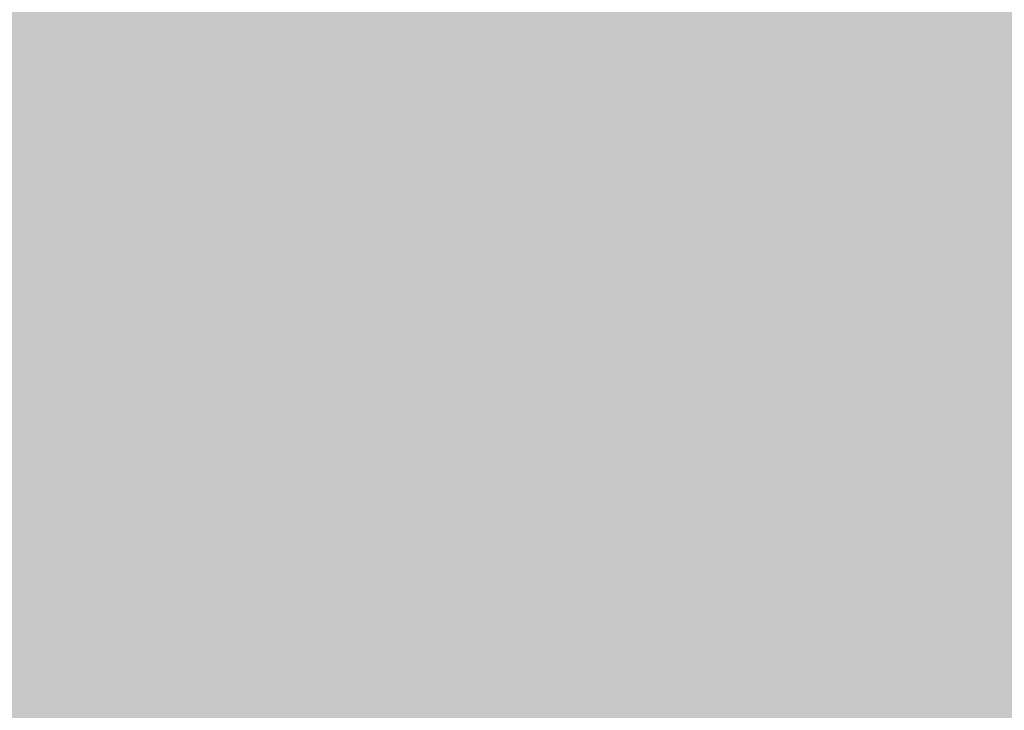
# Model space of a CAD drawing. Units: inches. Extents: x 2091 to 2899, y 967 to 2217.
# Tile 171 of 256: x 2203.14684 to 2203.151632, y 1152.250422 to 1152.253784. Entities that reach past the tile are written whole.
import ezdxf

# ---------------------------------------------------------------- set-up
doc = ezdxf.new("R2010")
doc.units = ezdxf.units.IN
doc.layers.add('A-WALL-PATT', color=141, linetype='Continuous', lineweight=13, true_color=0xadddf7)

msp = doc.modelspace()

# ---------------------------------------------------------------- hatches: boundary and pattern name
at = {"layer": 'A-WALL-PATT'}
h = msp.add_hatch(color=256, dxfattribs=at)
h.dxf.hatch_style = 1
h.paths.add_polyline_path([(2803.1436027, 2050.9190588), (2203.1436027, 2050.9190588), (2203.1436027, 1090.9190588), (2803.1436027, 1090.9190588)])
h.paths.add_polyline_path([(2635.7988501, 1147.5404649), (2674.5240524, 1147.5404649, 0.376086), (2678.5296653, 1152.8802017), (2678.5296653, 1159.5564734, 0.333335), (2674.524319, 1163.561846), (2674.524319, 1163.5618504), (2674.524319, 1192.9343904), (2635.8059707, 1192.9343904), (2597.0876225, 1192.9343904), (2597.0876225, 1163.561846, 0.333335), (2593.0822761, 1159.5564734), (2593.0822761, 1152.8802017, 0.376086), (2597.087889, 1147.5404649)], flags=0)
h.paths.add_polyline_path([(2436.0104329, 1278.2407784, 0.000483), (2435.9526433, 1278.215027, -0.001328), (2435.9356253, 1278.1116934, -0.001711), (2436.1164401, 1278.0407583, 0.002185)], flags=0)
h.paths.add_polyline_path([(2794.1436027, 1143.4190588), (2794.1436027, 1347.4190588), (2543.3701706, 1347.4190588), (2543.3701706, 1351.9190588), (2794.1436027, 1351.9190588), (2794.1436027, 1392.7135549), (2793.9473982, 1392.7135549), (2793.9473982, 1473.5368999), (2794.1436027, 1473.5368999), (2794.1436027, 1531.9190588), (2650.1436027, 1531.9190588), (2650.1436027, 1536.4190588), (2794.1436027, 1536.4190588), (2794.1436027, 1692.4190588), (2609.3756095, 1692.4190588), (2609.3756095, 1644.4190588), (2604.8756095, 1644.4190588), (2604.8756095, 1744.9190588), (2609.3756095, 1744.9190588), (2609.3756095, 1696.9190588), (2794.1436027, 1696.9190588), (2794.1436027, 1780.9190588), (2609.6436027, 1780.9190588), (2493.8756095, 1780.9190588), (2493.8756095, 1785.4190588), (2609.6436027, 1785.4190588), (2794.1436027, 1785.4190588), (2794.1436027, 1847.9388214), (2793.9512217, 1847.9388214), (2793.9512217, 1928.7621663), (2794.1436027, 1928.7621663), (2794.1436027, 1941.4190588), (2614.1436027, 1941.4190588), (2614.1436027, 1821.4190588), (2609.6436027, 1821.4190588), (2609.6436027, 1941.4190588), (2392.1436027, 1941.4190588), (2392.1436027, 1819.9190588), (2387.6436027, 1819.9190588), (2387.6436027, 1941.4190588), (2212.1436027, 1941.4190588), (2212.1436027, 1783.9190588), (2392.1436027, 1783.9190588), (2392.1436027, 1780.9190588), (2212.1436027, 1780.9190588), (2212.1436027, 1629.4190588), (2387.6436027, 1629.4190588), (2387.6436027, 1744.9190588), (2392.1436027, 1744.9190588), (2392.1436027, 1627.9190588), (2317.1436027, 1627.9190588), (2317.1436027, 1551.4190588), (2317.1436027, 1536.4190588), (2459.3835909, 1536.4190588), (2459.3835909, 1602.3964802), (2463.8835909, 1602.3964802), (2463.8835909, 1531.9190588), (2456.6436027, 1531.9190588), (2456.6436027, 1529.9190588), (2452.1436027, 1529.9190588), (2452.1436027, 1531.9190588), (2312.6436027, 1531.9190588), (2312.6436027, 1551.4190588), (2306.1436027, 1551.4190588), (2306.1436027, 1555.9190588), (2308.1436027, 1555.9190588), (2308.1436027, 1551.4190588), (2312.6436027, 1551.4190588), (2312.6436027, 1627.9190588), (2212.1436027, 1627.9190588), (2212.1436027, 1555.9190588), (2270.1436027, 1555.9190588), (2270.1436027, 1551.4190588), (2212.1436027, 1551.4190588), (2212.1436027, 1351.9190588), (2272.1436027, 1351.9190588), (2272.1436027, 1347.4190588), (2212.1436027, 1347.4190588), (2212.1436027, 1275.4190588), (2308.1436027, 1275.4190588), (2308.1436027, 1351.9190588), (2452.1436027, 1351.9190588), (2452.1436027, 1493.9190588), (2456.6436027, 1493.9190588), (2456.6436027, 1347.4190588), (2312.6436027, 1347.4190588), (2312.6436027, 1270.9190588), (2212.1436027, 1270.9190588), (2212.1436027, 1099.9190588), (2281.2375229, 1099.9190588), (2282.8710413, 1110.9138034), (2282.0083413, 1116.9966034), (2278.5577413, 1121.4204034), (2268.2056413, 1128.0562034), (2272.0876413, 1128.0562034), (2273.8129413, 1131.9270034), (2279.4203413, 1134.6919034), (2285.0278413, 1135.2449034), (2287.6158413, 1137.4568034), (2288.0471413, 1138.0098034), (2289.3411413, 1140.7747034), (2291.0665413, 1139.6687034), (2292.3605413, 1135.2449034), (2295.3798413, 1136.9038034), (2296.2425413, 1135.7979034), (2297.1052413, 1133.0330034), (2300.1246413, 1138.0098034), (2303.1439413, 1138.0098034), (2304.4379413, 1135.7979034), (2303.1439413, 1133.5860034), (2306.5946413, 1134.6919034), (2307.8887413, 1133.0330034), (2310.9080413, 1135.2449034), (2313.9274413, 1134.1389034), (2315.6268599, 1132.4271023), (2308.3200413, 1117.5496034), (2290.2038413, 1109.8079034), (2288.9098413, 1103.1721034), (2289.2723086, 1099.9190588), (2434.9182274, 1099.9190588), (2431.5932274, 1124.7880588), (2429.9302274, 1169.5530588), (2430.9271848, 1240.5196942), (2435.6589255, 1238.1861258), (2437.1352274, 1196.5540588), (2438.7982274, 1143.9730588), (2442.6782274, 1111.9980588), (2446.5582274, 1099.9190588), (2794.1436027, 1099.9190588), (2794.1436027, 1138.9190588), (2548.0324471, 1138.9190588), (2548.0324471, 1143.4190588), (2548.0324471, 1148.8190588), (2546.6684571, 1148.0315588), (2528.6856919, 1179.1786218, 0.256256), (2512.0324471, 1148.8190588), (2512.0324471, 1143.4190588), (2512.0324471, 1138.9190588), (2507.5324471, 1138.9190588), (2507.5324471, 1143.4190588), (2507.5324471, 1148.8190588, 0.256256), (2490.8792023, 1179.1786218), (2472.8964371, 1148.0315588), (2471.5324471, 1148.8190588), (2471.5324471, 1143.4190588), (2467.0324471, 1143.4190588), (2467.0324471, 1269.9457858, 0.039061), (2460.9099871, 1273.5800588), (2467.0324471, 1273.5800588), (2467.0324471, 1286.3253638, 0.014511), (2465.2161944, 1286.7619052), (2467.0324471, 1287.0525761), (2467.0324471, 1323.4190588), (2471.5324471, 1323.4190588), (2471.5324471, 1148.8190588), (2489.5324471, 1179.9959734), (2490.8964371, 1179.2084734), (2490.8792023, 1179.1786218, -0.256256), (2507.5324471, 1148.8190588), (2507.5324471, 1143.4190588), (2512.0324471, 1143.4190588), (2512.0324471, 1148.8190588, -0.256256), (2528.6856919, 1179.1786218), (2528.6684571, 1179.2084734), (2530.0324471, 1179.9959734), (2548.0324471, 1148.8190588), (2548.0324471, 1143.4190588)], flags=16)
h.paths.add_polyline_path([(2607.7685461, 1200.9450832), (2607.7685461, 1265.0306251), (2597.0876225, 1281.0520106), (2619.7845852, 1281.0520106), (2627.795278, 1337.1268598), (2635.7988501, 1337.1268598), (2643.8166634, 1337.1268598), (2651.8273562, 1281.0520106), (2674.524319, 1281.0520106), (2663.8433953, 1265.0306251), (2663.8433953, 1200.9450832), (2635.8059707, 1200.9450832)], flags=0)
edge = h.paths.add_edge_path(flags=0)
edge.add_ellipse((13303.8962153, 1272.9987247), major_axis=(-10595.3130399, 0.0000005), ratio=0.842303870086, start_angle=0.62823721906, end_angle=0.64655409989, ccw=False)
edge.add_ellipse((2711.7004495, 1156.8526781), major_axis=(2.2197691, 0), ratio=0.84230387, start_angle=111.5352435, end_angle=180.6282372, ccw=False)
edge.add_ellipse((13303.1562922, 1272.9987246), major_axis=(-10593.0263064, 0), ratio=0.842303869544, start_angle=0.52827147182, end_angle=0.64655409706, ccw=False)
edge.add_line((2710.7645961, 1175.3332951), (2710.1299858, 1175.3332951))
edge.add_ellipse((2710.1299858, 1176.5797752), major_axis=(1.4798461, 0), ratio=0.84230387, start_angle=180, end_angle=270, ccw=False)
edge.add_line((2708.6501397, 1176.5797752), (2708.6501397, 1200.7829144))
edge.add_ellipse((2710.1299858, 1200.7829144), major_axis=(1.4798461, 0), ratio=0.84230387, start_angle=90, end_angle=180, ccw=False)
edge.add_line((2710.1299858, 1202.0293944), (2710.4650752, 1202.0293944))
edge.add_ellipse((13303.1562922, 1272.9987246), major_axis=(-10593.0263064, 0), ratio=0.842303869544, start_angle=-0.09022908859, end_angle=0.38386677879, ccw=False)
edge.add_ellipse((2710.1299858, 1290.9270308), major_axis=(-1.4798461, 0), ratio=0.84230387, start_angle=0, end_angle=90, ccw=False)
edge.add_line((2708.6501397, 1290.9270308), (2708.6501397, 1315.13017))
edge.add_ellipse((2710.1299858, 1315.13017), major_axis=(-1.4798461, 0), ratio=0.84230387, start_angle=-90, end_angle=0, ccw=False)
edge.add_line((2710.1299858, 1316.3766501), (2710.7063141, 1316.3766501))
edge.add_ellipse((3238.4017202, 1296.2895655), major_axis=(528.2339998, 0), ratio=0.84230386954, start_angle=176.349572414, end_angle=177.820049686, ccw=False)
edge.add_ellipse((2775.0630432, 1071.4506962), major_axis=(313.3077613, 0), ratio=0.84230386954, start_angle=102.125965552, end_angle=103.780528989, ccw=False)
edge.add_ellipse((2775.0630432, 1078.3056979), major_axis=(-305.3028915, 0), ratio=0.84230386955, start_angle=-79.790461003, end_angle=-77.555372706, ccw=False)
edge.add_ellipse((2695.1417666, 1541.9753825), major_axis=(-250.9602162, 0), ratio=0.84230386954, start_angle=99.256566007, end_angle=102.554932644)
edge.add_line((2741.4103262, 1334.2142554), (2747.1325454, 1337.3784768))
edge.add_ellipse((2747.5386163, 1336.8574776), major_axis=(-0.739923, 0), ratio=0.84230387, start_angle=270, end_angle=307.9331305, ccw=False)
edge.add_ellipse((2747.5386163, 1336.8574776), major_axis=(-0.739923, 0), ratio=0.84230387, start_angle=232.0668695, end_angle=270, ccw=False)
edge.add_line((2747.9446872, 1337.3784768), (2753.6669064, 1334.2142554))
edge.add_ellipse((2799.935466, 1541.9753825), major_axis=(250.9602162, 0), ratio=0.84230386954, start_angle=257.445067356, end_angle=260.743433993)
edge.add_ellipse((2720.0141894, 1078.3056979), major_axis=(305.3028915, 0), ratio=0.84230386954, start_angle=77.555372707, end_angle=79.790461003, ccw=False)
edge.add_ellipse((2720.0141894, 1071.4506962), major_axis=(-313.3077613, 0), ratio=0.84230386954, start_angle=256.219471011, end_angle=257.874034448, ccw=False)
edge.add_ellipse((2256.6755124, 1296.2895655), major_axis=(-528.2339998, 0), ratio=0.84230386954, start_angle=182.179950314, end_angle=183.650427586, ccw=False)
edge.add_line((2784.3709184, 1316.3766501), (2784.9472468, 1316.3766501))
edge.add_ellipse((2784.9472468, 1315.13017), major_axis=(1.4798461, 0), ratio=0.84230387, start_angle=0, end_angle=90, ccw=False)
edge.add_line((2786.4270928, 1315.13017), (2786.4270928, 1290.9270308))
edge.add_ellipse((2784.9472468, 1290.9270308), major_axis=(1.4798461, 0), ratio=0.84230387, start_angle=270, end_angle=360, ccw=False)
edge.add_ellipse((-7808.0790596, 1272.9987246), major_axis=(10593.0263063, 0), ratio=0.842303869544, start_angle=-0.38386677879, end_angle=0.09022908859, ccw=False)
edge.add_line((2784.6121574, 1202.0293944), (2784.9472468, 1202.0293944))
edge.add_ellipse((2784.9472468, 1200.7829144), major_axis=(1.4798461, 0), ratio=0.84230387, start_angle=0, end_angle=90, ccw=False)
edge.add_line((2786.4270928, 1200.7829144), (2786.4270928, 1176.5797752))
edge.add_ellipse((2784.9472468, 1176.5797752), major_axis=(-1.4798461, 0), ratio=0.84230387, start_angle=90, end_angle=180, ccw=False)
edge.add_line((2784.9472468, 1175.3332951), (2784.3126365, 1175.3332951))
edge.add_ellipse((-7808.0790596, 1272.9987246), major_axis=(10593.0263063, 0), ratio=0.842303869544, start_angle=-0.61864319632, end_angle=-0.52827147182, ccw=False)
edge.add_ellipse((2783.3767831, 1156.8526781), major_axis=(-2.2197691, 0), ratio=0.84230387, start_angle=179.3717628, end_angle=248.4647566, ccw=False)
edge.add_ellipse((-7808.8189826, 1272.9987246), major_axis=(-10595.3130398, 0.0000036), ratio=0.842303865762, start_angle=179.3534459226, end_angle=179.37176280343, ccw=False)
edge.add_ellipse((2780.2973026, 1153.500793), major_axis=(-5.2464256, 0), ratio=0.84230387, start_angle=90, end_angle=179.3534459, ccw=False)
edge.add_line((2780.2973026, 1149.0817084), (2714.77993, 1149.0817084))
edge.add_ellipse((2714.77993, 1153.500793), major_axis=(5.2464256, 0), ratio=0.84230387, start_angle=180.6465541, end_angle=270, ccw=False)
edge = h.paths.add_edge_path(flags=0)
edge.add_line((2718.1873674, 1151.0078329), (2718.1873674, 1170.4723638))
edge.add_ellipse((2721.1470595, 1170.4723638), major_axis=(-2.9596921, 0), ratio=0.84230387, start_angle=-90, end_angle=0, ccw=False)
edge.add_line((2721.1470595, 1172.965324), (2773.9301731, 1172.965324))
edge.add_ellipse((2773.9301731, 1170.4723638), major_axis=(-2.9596921, 0), ratio=0.84230387, start_angle=180, end_angle=270, ccw=False)
edge.add_line((2776.8898652, 1170.4723638), (2776.8898652, 1151.0078329))
edge.add_line((2776.8898652, 1151.0078329), (2718.1873674, 1151.0078329))
edge = h.paths.add_edge_path(flags=0)
edge.add_line((2718.1873674, 1180.2341502), (2718.1873674, 1199.0578342))
edge.add_ellipse((2747.5386163, 1320.3986402), major_axis=(147.0179239, 0), ratio=0.84230386954, start_angle=256.40186531, end_angle=283.59813469)
edge.add_line((2776.8898652, 1199.0578342), (2776.8898652, 1180.2341502))
edge.add_ellipse((2747.5386163, 1301.5749562), major_axis=(147.0179239, 0), ratio=0.84230386954, start_angle=256.40186531, end_angle=283.59813469, ccw=False)
edge = h.paths.add_edge_path(flags=0)
edge.add_ellipse((13303.1562922, 1272.9987246), major_axis=(-10591.5464603, 0), ratio=0.842303869555, start_angle=0.05559431352, end_angle=0.37776419393, ccw=False)
edge.add_line((2711.6168595, 1262.7217103), (2715.6674076, 1249.4953957))
edge.add_ellipse((6413.8919626, 1241.691919), major_axis=(-3698.2361592, 0), ratio=0.842303869547, start_angle=-0.120897369, end_angle=0.3640763489)
edge.add_line((2715.7610383, 1218.1924547), (2711.9343065, 1203.167361))
edge = h.paths.add_edge_path(flags=0)
edge.add_line((2718.1873674, 1251.074566), (2716.0024854, 1267.4504351))
edge.add_ellipse((2742.1511746, 1202.1895399), major_axis=(81.7725845, 0), ratio=0.8423038695, start_angle=94.277420963, end_angle=111.834953797, ccw=False)
edge.add_line((2737.0097482, 1270.9306255), (2758.0674844, 1270.9306255))
edge.add_ellipse((2752.926058, 1202.1895399), major_axis=(81.7725845, 0), ratio=0.8423038695, start_angle=68.165046203, end_angle=85.722579037, ccw=False)
edge.add_line((2779.0747472, 1267.4504351), (2776.8898652, 1251.074566))
edge.add_ellipse((2750.3380588, 1187.8853558), major_axis=(79.5796641, 0), ratio=0.8423038695, start_angle=67.208085122, end_angle=85.129930403)
edge.add_line((2756.0346562, 1254.7436557), (2739.0425764, 1254.7436557))
edge.add_ellipse((2744.7391738, 1187.8853558), major_axis=(79.5796641, 0), ratio=0.8423038695, start_angle=94.870069597, end_angle=112.791914878)
edge = h.paths.add_edge_path(flags=0)
edge.add_line((2783.1429261, 1203.167361), (2779.3161943, 1218.1924547))
edge.add_ellipse((-918.81473, 1241.691919), major_axis=(3698.2361592, 0), ratio=0.842303869546, start_angle=-0.3640763489, end_angle=0.120897369)
edge.add_line((2779.409825, 1249.4953957), (2783.4603731, 1262.7217103))
edge.add_ellipse((-7808.0790596, 1272.9987246), major_axis=(-10591.5464603, 0), ratio=0.84230386954, start_angle=179.6222358061, end_angle=179.94440568651, ccw=False)
edge = h.paths.add_edge_path(flags=0)
edge.add_ellipse((2734.2008921, 1286.6904402), major_axis=(-0.3566086, 6.3400775), ratio=0.603833576, start_angle=89.00201428, end_angle=253.65740805, ccw=False)
edge.add_line((2730.3690013, 1286.5418057), (2730.3690013, 1301.3519803))
edge.add_line((2730.3690013, 1301.3519803), (2735.9133107, 1305.2148028))
edge.add_ellipse((2736.3849168, 1304.7345612), major_axis=(0.739923, 0), ratio=0.84230387, start_angle=90, end_angle=134.4802109, ccw=False)
edge.add_line((2736.3849168, 1305.3578013), (2738.0327829, 1305.3578013))
edge.add_line((2738.0327829, 1305.3578013), (2738.0327829, 1307.7079274))
edge.add_ellipse((2794.201642, 1307.7079274), major_axis=(56.168859, 0), ratio=0.8423038695, start_angle=150.5614304, end_angle=180, ccw=False)
edge.add_ellipse((2700.8755906, 1307.7079274), major_axis=(-56.168859, 0), ratio=0.8423038695, start_angle=180, end_angle=209.4385696, ccw=False)
edge.add_line((2757.0444497, 1307.7079274), (2757.0444497, 1305.3578013))
edge.add_line((2757.0444497, 1305.3578013), (2758.6923157, 1305.3578013))
edge.add_ellipse((2758.6923157, 1304.7345612), major_axis=(-0.739923, 0), ratio=0.84230387, start_angle=225.5197891, end_angle=270, ccw=False)
edge.add_line((2759.1639219, 1305.2148028), (2764.7082312, 1301.3519803))
edge.add_line((2764.7082312, 1301.3519803), (2764.7082312, 1286.5418057))
edge.add_ellipse((2760.8763405, 1286.6904402), major_axis=(0.3566086, 6.3400775), ratio=0.603833576, start_angle=106.34259195, end_angle=270.99798572, ccw=False)
edge.add_line((2757.0444497, 1285.7970896), (2757.0444497, 1307.7079274))
edge.add_ellipse((2700.8755906, 1307.7079274), major_axis=(-56.168859, 0), ratio=0.8423038695, start_angle=180, end_angle=209.4385696)
edge.add_ellipse((2794.201642, 1307.7079274), major_axis=(56.168859, 0), ratio=0.8423038695, start_angle=150.5614304, end_angle=180)
edge.add_line((2738.0327829, 1307.7079274), (2738.0327829, 1285.7970896))
h.paths.add_polyline_path([(2417.8122727, 1104.449704), (2413.4922727, 1102.529704), (2410.6122727, 1103.969704), (2409.1722727, 1106.369704), (2407.2522727, 1107.329704), (2406.2922727, 1109.729704), (2405.3322727, 1114.049704), (2405.3322727, 1117.889704), (2406.2922727, 1120.129704), (2407.2522727, 1119.809704), (2408.8483218, 1118.3276585), (2410.1739451, 1119.4241703), (2410.2112727, 1120.405704), (2411.0407305, 1121.4190541), (2410.6992727, 1119.858704), (2410.1739451, 1119.4241703), (2410.0884515, 1117.1761095), (2411.1328361, 1116.2063237), (2413.9722727, 1119.329704), (2416.8522727, 1120.769704), (2416.8697209, 1120.7987842), (2417.0350713, 1119.4051162), (2417.8962134, 1118.1433844), (2418.2922727, 1118.369704), (2419.5444467, 1120.0392692), (2419.3609153, 1118.387487), (2419.0321078, 1119.3561507), (2418.3989394, 1118.5119262), (2419.2522727, 1114.529704), (2418.7940909, 1107.1987949)], flags=0)
h.paths.add_polyline_path([(2508.8701706, 1347.4190588), (2508.3701706, 1347.4190588), (2508.3701706, 1351.9190588), (2508.8701706, 1351.9190588)], flags=0)
h.paths.add_polyline_path([(2473.3701706, 1347.4190588), (2472.3701706, 1347.4190588), (2467.8701706, 1347.4190588), (2467.8701706, 1455.4190588), (2472.3701706, 1455.4190588), (2472.3701706, 1352.4190588), (2473.3701706, 1352.4190588)], flags=0)
h.paths.add_polyline_path([(2352.106244, 1217.4461971), (2349.226244, 1218.8861971), (2347.786244, 1221.2861971), (2345.866244, 1222.2461971), (2344.906244, 1224.6461971), (2343.946244, 1228.9661971), (2343.946244, 1232.8061971), (2344.906244, 1235.0461971), (2345.866244, 1234.7261971), (2347.4622931, 1233.2441515), (2348.7879164, 1234.3406634), (2348.825244, 1235.3221971), (2349.6547018, 1236.3355471), (2349.313244, 1234.7751971), (2348.7879164, 1234.3406634), (2348.7024228, 1232.0926025), (2349.7468074, 1231.1228168), (2352.586244, 1234.2461971), (2355.466244, 1235.6861971), (2355.4836921, 1235.7152773), (2355.6490426, 1234.3216093), (2356.5101846, 1233.0598774), (2356.906244, 1233.2861971), (2358.1584179, 1234.9557623), (2357.9748866, 1233.3039801), (2357.6460791, 1234.2726438), (2357.0129107, 1233.4284193), (2357.866244, 1229.4461971), (2357.4080622, 1222.115288), (2356.426244, 1219.3661971)], flags=0)
h.paths.add_polyline_path([(2348.2967999, 1112.2244204), (2347.0137999, 1112.3104204), (2345.5297999, 1114.1274204), (2345.7317999, 1115.8584204), (2346.8117999, 1116.9824204), (2346.8117999, 1114.6464204), (2345.8667999, 1114.2144204), (2346.8797999, 1114.3004204)], flags=0)
h.paths.add_polyline_path([(2347.0137999, 1110.9264204), (2346.2717999, 1110.4934204), (2346.6097999, 1111.1864204)], flags=0)
h.paths.add_polyline_path([(2345.8667999, 1118.1944204), (2345.5297999, 1117.3294204), (2343.7077999, 1118.0214204), (2344.3827999, 1118.6264204)], flags=0)
h.paths.add_polyline_path([(2346.6767999, 1109.2824204), (2346.0697999, 1108.0714204), (2345.8667999, 1110.0614204)], flags=0)
h.paths.add_polyline_path([(2345.0567999, 1119.7514204), (2343.6397999, 1119.7514204), (2343.9777999, 1121.1354204)], flags=0)
h.paths.add_polyline_path([(2345.2597999, 1116.5504204), (2345.1247999, 1115.8584204), (2344.9217999, 1115.6854204), (2344.7197999, 1116.3774204)], flags=0)
h.paths.add_polyline_path([(2345.6647999, 1112.3104204), (2345.4617999, 1111.5324204), (2344.0447999, 1111.9644204), (2344.6517999, 1112.5704204)], flags=0)
h.paths.add_polyline_path([(2345.1917999, 1113.3494204), (2344.4497999, 1113.8684204), (2344.7197999, 1114.3874204)], flags=0)
h.paths.add_polyline_path([(2344.6517999, 1116.8094204), (2344.1797999, 1115.6854204), (2344.6517999, 1115.3394204), (2343.9097999, 1114.9064204), (2343.0327999, 1115.9444204), (2343.6397999, 1116.4634204)], flags=0)
h.paths.add_polyline_path([(2345.8667999, 1106.6864204), (2344.9897999, 1105.5624204), (2344.5167999, 1106.6004204)], flags=0)
h.paths.add_polyline_path([(2344.8547999, 1110.0614204), (2344.5167999, 1109.2824204), (2344.1127999, 1109.7154204)], flags=0)
h.paths.add_polyline_path([(2344.0447999, 1113.5224204), (2343.4377999, 1113.0894204), (2342.7627999, 1113.9544204)], flags=0)
h.paths.add_polyline_path([(2344.3147999, 1111.0124204), (2342.9647999, 1110.3204204), (2342.9647999, 1111.0994204)], flags=0)
h.paths.add_polyline_path([(2345.1247999, 1104.6974204), (2344.5847999, 1103.7454204), (2344.4497999, 1104.2644204)], flags=0)
h.paths.add_polyline_path([(2342.8297999, 1121.2224204), (2341.7497999, 1120.5304204), (2340.5357999, 1121.0494204), (2340.1307999, 1121.8284204), (2340.6707999, 1122.9524204), (2341.1427999, 1121.8284204), (2341.6147999, 1122.0014204)], flags=0)
h.paths.add_polyline_path([(2342.9647999, 1119.7514204), (2343.0327999, 1118.4534204), (2342.0877999, 1118.0214204), (2342.0197999, 1119.4914204)], flags=0)
h.paths.add_polyline_path([(2342.6947999, 1116.8964204), (2341.9527999, 1116.6364204), (2342.0197999, 1117.3294204)], flags=0)
h.paths.add_polyline_path([(2343.0327999, 1112.2244204), (2342.0197999, 1111.7914204), (2341.5477999, 1112.2244204), (2342.3577999, 1113.3494204)], flags=0)
h.paths.add_polyline_path([(2343.7747999, 1104.4374204), (2342.6277999, 1102.8804204), (2342.6947999, 1104.6104204), (2343.4377999, 1105.1294204)], flags=0)
h.paths.add_polyline_path([(2342.0197999, 1115.0794204), (2340.8057999, 1115.5124204), (2340.9407999, 1116.3774204)], flags=0)
h.paths.add_polyline_path([(2341.4807999, 1120.0974204), (2341.4807999, 1119.4054204), (2341.0757999, 1119.5784204), (2341.1427999, 1120.0974204)], flags=0)
h.paths.add_polyline_path([(2341.8177999, 1114.4734204), (2340.9407999, 1113.0894204), (2340.8057999, 1114.5604204)], flags=0)
h.paths.add_polyline_path([(2341.1427999, 1118.5404204), (2340.9407999, 1116.9824204), (2339.0507999, 1117.6754204), (2339.0507999, 1118.6264204)], flags=0)
h.paths.add_polyline_path([(2342.6947999, 1101.6684204), (2341.9527999, 1101.8414204), (2342.5597999, 1102.3614204)], flags=0)
h.paths.add_polyline_path([(2340.3327999, 1119.6654204), (2338.4437999, 1119.5784204), (2337.9037999, 1120.3574204), (2339.6577999, 1120.6164204)], flags=0)
h.paths.add_polyline_path([(2340.3327999, 1115.3394204), (2340.0627999, 1113.6954204), (2339.3877999, 1115.3394204)], flags=0)
h.paths.add_polyline_path([(2341.8177999, 1103.8314204), (2341.5477999, 1102.8804204), (2341.1427999, 1103.6584204)], flags=0)
h.paths.add_polyline_path([(2339.0507999, 1122.8664204), (2337.2957999, 1121.8284204), (2337.0937999, 1123.1254204), (2337.7687999, 1123.8184204)], flags=0)
h.paths.add_polyline_path([(2339.1177999, 1121.7414204), (2338.8477999, 1121.2224204), (2338.1737999, 1121.0494204), (2338.3757999, 1121.5684204)], flags=0)
h.paths.add_polyline_path([(2339.1857999, 1119.3194204), (2338.6457999, 1118.7134204), (2338.2407999, 1118.1074204), (2338.2407999, 1118.8864204)], flags=0)
h.paths.add_polyline_path([(2341.1427999, 1101.9284204), (2340.6027999, 1101.2364204), (2340.0627999, 1101.8414204), (2340.6027999, 1102.3614204)], flags=0)
h.paths.add_polyline_path([(2337.6337999, 1117.7614204), (2336.6207999, 1118.2804204), (2337.2957999, 1118.9724204)], flags=0)
h.paths.add_polyline_path([(2336.8237999, 1119.5784204), (2334.7987999, 1118.9724204), (2335.2037999, 1120.3574204), (2336.5537999, 1120.8764204)], flags=0)
h.paths.add_polyline_path([(2339.1177999, 1100.4574204), (2337.3637999, 1100.5434204), (2336.7557999, 1101.2364204)], flags=0)
h.paths.add_polyline_path([(2336.3507999, 1122.4334204), (2336.0137999, 1121.9144204), (2334.9337999, 1122.4334204), (2334.5287999, 1123.4714204), (2335.7437999, 1122.7794204)], flags=0)
h.paths.add_polyline_path([(2334.7317999, 1120.8764204), (2334.2587999, 1120.3574204), (2334.0567999, 1120.7894204), (2334.5967999, 1121.3084204)], flags=0)
h.paths.add_polyline_path([(2334.4617999, 1122.1744204), (2332.5717999, 1121.3084204), (2331.3567999, 1122.1744204), (2332.0997999, 1122.8664204)], flags=0)
h.paths.add_polyline_path([(2334.2587999, 1118.5404204), (2333.3817999, 1118.4534204), (2333.6517999, 1119.3194204)], flags=0)
h.paths.add_polyline_path([(2335.5417999, 1102.2744204), (2334.1917999, 1102.6204204), (2335.2717999, 1103.3124204)], flags=0)
h.paths.add_polyline_path([(2332.7067999, 1119.6654204), (2331.6947999, 1120.4434204), (2332.5047999, 1120.7894204)], flags=0)
h.paths.add_polyline_path([(2334.7317999, 1101.1494204), (2333.5167999, 1101.5824204), (2333.9887999, 1101.7554204)], flags=0)
h.paths.add_polyline_path([(2332.6397999, 1116.6364204), (2331.0867999, 1116.2904204), (2331.9647999, 1118.1944204)], flags=0)
h.paths.add_polyline_path([(2330.7497999, 1121.5684204), (2330.2767999, 1120.2704204), (2328.5227999, 1119.3194204), (2328.9947999, 1121.0494204)], flags=0)
h.paths.add_polyline_path([(2330.7497999, 1118.6264204), (2330.0077999, 1117.5024204), (2329.8727999, 1118.0214204)], flags=0)
h.paths.add_polyline_path([(2332.0997999, 1102.3614204), (2330.5467999, 1102.0144204), (2331.6947999, 1102.9664204)], flags=0)
h.paths.add_polyline_path([(2329.5347999, 1113.6084204), (2329.0627999, 1112.3104204), (2328.5897999, 1113.3494204)], flags=0)
h.paths.add_polyline_path([(2328.3877999, 1117.8484204), (2327.5097999, 1116.5504204), (2327.1727999, 1117.7614204)], flags=0)
h.paths.add_polyline_path([(2329.7377999, 1106.5134204), (2329.5347999, 1105.3024204), (2328.2527999, 1106.0814204)], flags=0)
h.paths.add_polyline_path([(2328.6577999, 1114.3874204), (2328.0497999, 1114.1274204), (2328.3197999, 1114.9064204)], flags=0)
h.paths.add_polyline_path([(2328.3197999, 1112.2244204), (2327.1057999, 1112.1374204), (2326.7007999, 1112.6564204)], flags=0)
h.paths.add_polyline_path([(2326.9027999, 1115.2524204), (2326.7007999, 1114.1274204), (2325.2157999, 1113.6084204), (2326.0927999, 1115.3394204)], flags=0)
h.paths.add_polyline_path([(2326.6327999, 1108.3304204), (2326.0927999, 1107.3794204), (2325.8907999, 1108.5034204), (2326.4977999, 1109.1094204)], flags=0)
h.paths.add_polyline_path([(2615.1436027, 1531.9190588), (2609.6436027, 1531.9190588), (2609.6436027, 1620.4190588), (2614.1436027, 1620.4190588), (2614.1436027, 1536.4190588), (2615.1436027, 1536.4190588)], flags=0)
h.paths.add_polyline_path([(2545.1436027, 1563.4190588), (2464.1436027, 1563.4190588), (2464.1436027, 1632.4190588), (2509.1436027, 1632.4190588), (2509.1436027, 1627.9190588), (2509.1436027, 1603.9190588), (2468.6436027, 1603.9190588), (2468.6436027, 1567.9190588), (2540.6436027, 1567.9190588), (2540.6436027, 1591.9190588), (2545.1436027, 1591.9190588)], flags=0)
h.paths.add_polyline_path([(2388.9690483, 1549.985735), (2357.4341811, 1549.985735), (2357.4341811, 1623.3607783), (2399.3627772, 1623.3607783), (2435.6894654, 1623.3607783), (2435.5925469, 1602.5592734), (2435.5925469, 1602.3964802), (2388.9690483, 1602.3964802)], flags=0)
h.paths.add_polyline_path([(2388.8806282, 1555.8091511), (2374.9044295, 1555.8091511), (2374.9044295, 1600.5715641), (2374.9044295, 1615.4576454), (2406.3508766, 1615.4576454), (2406.3508766, 1618.9394309), (2412.1742927, 1615.4576454), (2406.3508766, 1611.9758599), (2406.3508766, 1615.4576454), (2388.8806282, 1615.4576454)], flags=0)
h.paths.add_polyline_path([(2568.8756095, 1644.4190588), (2453.3756095, 1644.4190588), (2453.3756095, 1785.4190588), (2457.8756095, 1785.4190588), (2457.8756095, 1648.9190588), (2568.8756095, 1648.9190588)], flags=0)
h.paths.add_polyline_path([(2212.1436027, 1945.9190588), (2212.1436027, 2041.9190588), (2794.1436027, 2041.9190588), (2794.1436027, 1945.9190588)], flags=16)
h.paths.add_polyline_path([(2271.0827276, 1964.3172377), (2776.852968, 1964.3172377), (2776.852968, 2037.1696226), (2271.0827276, 2037.1696226)], flags=8)
h.paths.add_polyline_path([(2380.6492852, 1536.8241435), (2461.0408087, 1536.8241435), (2461.0408087, 1554.6525871), (2380.6492852, 1554.6525871)], flags=8)
h.paths.add_polyline_path([(2240.7557092, 1609.7254508), (2309.1858294, 1609.7254508), (2309.1858294, 1617.6982037), (2240.7557092, 1617.6982037)], flags=8)
h.paths.add_polyline_path([(2212.6772554, 1313.5041021), (2282.5915203, 1313.5041021), (2282.5915203, 1322.7452389), (2212.6772554, 1322.7452389)], flags=8)
h.paths.add_polyline_path([(2457.111976, 1114.778574), (2558.4815807, 1114.778574), (2558.4815807, 1142.2196823), (2457.111976, 1142.2196823)], flags=8)
h.paths.add_polyline_path([(2473.4423372, 1273.0100672), (2604.6412257, 1273.0100672), (2604.6412257, 1318.3469349), (2473.4423372, 1318.3469349)], flags=8)
h.paths.add_polyline_path([(2638.8763024, 1626.9774316), (2684.2503675, 1627.9767377), (2684.0384825, 1637.5974944), (2638.6644174, 1636.5981884)], flags=8)
h.paths.add_polyline_path([(2537.5905538, 1453.7934466), (2628.3895472, 1453.7934466), (2628.3895472, 1475.3448114), (2537.5905538, 1475.3448114)], flags=8)
h.paths.add_polyline_path([(2504.1376376, 1714.6323972), (2554.6471875, 1714.6323972), (2554.6471875, 1730.2377115), (2504.1376376, 1730.2377115)], flags=8)
h.paths.add_polyline_path([(2487.5011806, 1575.6518716), (2535.0971214, 1575.6518716), (2535.0971214, 1598.3776456), (2487.5011806, 1598.3776456)], flags=8)
h.paths.add_polyline_path([(2709.0994004, 1735.7102784), (2740.0166009, 1735.7102784), (2740.0166009, 1749.9376406), (2709.0994004, 1749.9376406)], flags=8)
h.paths.add_polyline_path([(2442.4384239, 1792.1716575), (2564.7288353, 1792.1716575), (2564.7288353, 1842.0001626), (2442.4384239, 1842.0001626)], flags=8)
h.paths.add_polyline_path([(2655.8158012, 1809.6440763), (2789.5201425, 1806.6937963), (2790.0849768, 1832.2916379), (2656.3806355, 1835.2419179)], flags=8)
h.paths.add_polyline_path([(2234.8426972, 1797.7201432), (2368.5928512, 1794.7688523), (2369.1607182, 1820.504132), (2235.4105642, 1823.4554229)], flags=8)
h.paths.add_polyline_path([(2245.1384659, 1644.0063348), (2398.4277329, 1640.6238997), (2398.9948417, 1666.3248199), (2245.7055747, 1669.7072549)], flags=8)
h.paths.add_polyline_path([(2306.1428474, 1431.1685186), (2413.7683138, 1428.7936873), (2414.3331481, 1454.3915289), (2306.7076817, 1456.7663602)], flags=8)
h.paths.add_polyline_path([(2306.834582, 1458.2331447), (2393.3804836, 1456.3234487), (2393.9328082, 1481.3543583), (2307.3869066, 1483.2640542)], flags=8)

doc.saveas('drawing.dxf')
